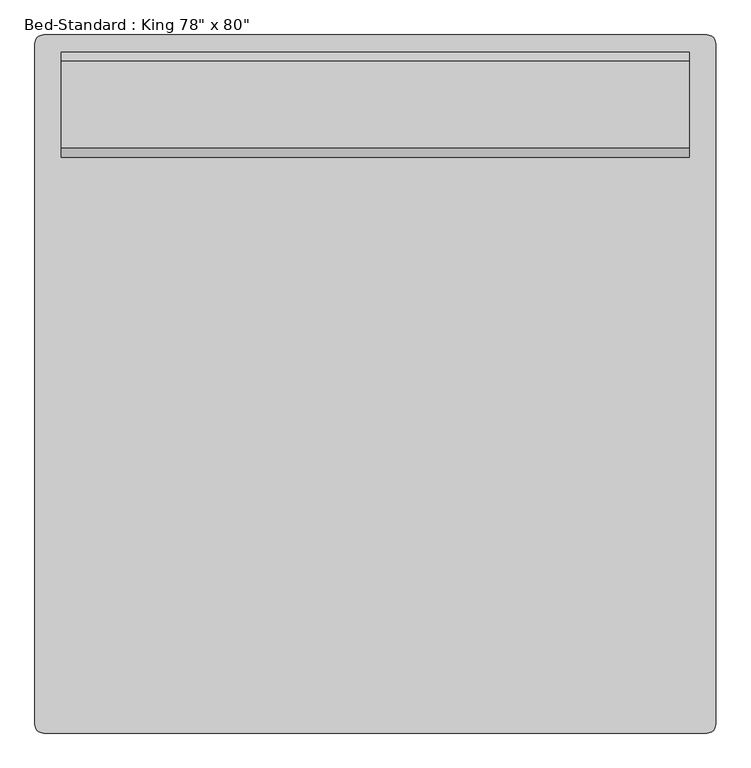
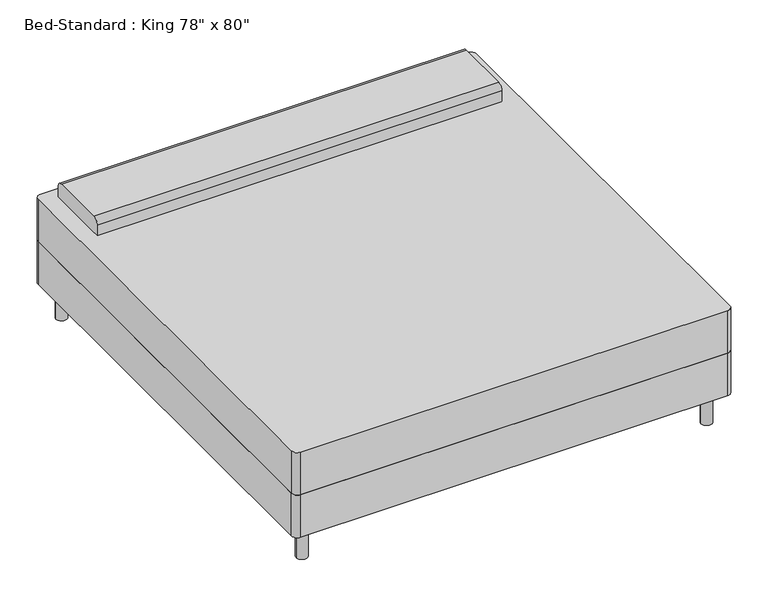
"""IFC4 building model written with IfcOpenShell, lengths in millimetres: furniture geometry."""

from ifc_helpers import new_model, si_unit, point, frame, frame_2d, origin, origin_with_axes, place, context, project, spatial, polyline, circle_curve, trimmed, segment, composite_curve, outline, extrude, source, transform, mapped, element, save


def furniture_1fc5af50(model_context):
    return source(origin(), model_context, "Body", "SweptSolid", [
        extrude(outline(composite_curve([segment(polyline([(-719.1114754, -1036.195082), (-719.1114754, 945.004918)]), True, "CONTINUOUS"), segment(trimmed(circle_curve(frame_2d((-693.7114754, 945.004918)), 25.4), [point((-719.1114754, 945.004918))], [point((-693.7114754, 970.404918))], False, "CARTESIAN"), True, "CONTINUOUS"), segment(polyline([(-693.7114754, 970.404918), (1236.6885246, 970.404918)]), True, "CONTINUOUS"), segment(trimmed(circle_curve(frame_2d((1236.6885246, 945.004918)), 25.4), [point((1236.6885246, 970.404918))], [point((1262.0885246, 945.004918))], False, "CARTESIAN"), True, "CONTINUOUS"), segment(polyline([(1262.0885246, 945.004918), (1262.0885246, -1036.195082)]), True, "CONTINUOUS"), segment(trimmed(circle_curve(frame_2d((1236.6885246, -1036.195082)), 25.4), [point((1262.0885246, -1036.195082))], [point((1236.6885246, -1061.595082))], False, "CARTESIAN"), True, "CONTINUOUS"), segment(polyline([(1236.6885246, -1061.595082), (-693.7114754, -1061.595082)]), True, "CONTINUOUS"), segment(trimmed(circle_curve(frame_2d((-693.7114754, -1036.195082)), 25.4), [point((-693.7114754, -1061.595082))], [point((-719.1114754, -1036.195082))], False, "CARTESIAN"), True, "CONTINUOUS")], self_intersect=False)), frame((0.0, 0.0, 152.4), z_axis=(0.0, 0.0, 1.0), x_axis=(1.0, 0.0, 0.0)), (0.0, 0.0, 1.0), 203.2),
        extrude(outline(composite_curve([segment(polyline([(614.804918, 558.8), (614.804918, 609.6)]), True, "CONTINUOUS"), segment(trimmed(circle_curve(frame_2d((640.204918, 609.6)), 25.4), [point((614.804918, 609.6))], [point((640.204918, 635.0))], False, "CARTESIAN"), True, "CONTINUOUS"), segment(polyline([(640.204918, 635.0), (894.204918, 635.0)]), True, "CONTINUOUS"), segment(trimmed(circle_curve(frame_2d((894.204918, 609.6)), 25.4), [point((894.204918, 635.0))], [point((919.604918, 609.6))], False, "CARTESIAN"), True, "CONTINUOUS"), segment(polyline([(919.604918, 609.6), (919.604918, 558.8), (614.804918, 558.8)]), True, "CONTINUOUS")], self_intersect=False)), frame((-642.9114754, 0.0, 0.0), z_axis=(1.0, 0.0, 0.0), x_axis=(0.0, 1.0, 0.0)), (0.0, 0.0, 1.0), 1828.8),
        extrude(outline(composite_curve([segment(trimmed(circle_curve(frame_2d((-642.9114754, 894.204918)), 25.4), [point((-668.3114754, 894.204918))], [point((-617.5114754, 894.204918))], False, "CARTESIAN"), True, "CONTINUOUS"), segment(trimmed(circle_curve(frame_2d((-642.9114754, 894.204918)), 25.4), [point((-617.5114754, 894.204918))], [point((-668.3114754, 894.204918))], False, "CARTESIAN"), True, "CONTINUOUS")], self_intersect=False)), origin_with_axes(), (0.0, 0.0, 1.0), 152.4),
        extrude(outline(composite_curve([segment(trimmed(circle_curve(frame_2d((1185.8885246, 894.204918)), 25.4), [point((1160.4885246, 894.204918))], [point((1211.2885246, 894.204918))], False, "CARTESIAN"), True, "CONTINUOUS"), segment(trimmed(circle_curve(frame_2d((1185.8885246, 894.204918)), 25.4), [point((1211.2885246, 894.204918))], [point((1160.4885246, 894.204918))], False, "CARTESIAN"), True, "CONTINUOUS")], self_intersect=False)), origin_with_axes(), (0.0, 0.0, 1.0), 152.4),
        extrude(outline(composite_curve([segment(trimmed(circle_curve(frame_2d((1185.8885246, -985.395082)), 25.4), [point((1160.4885246, -985.395082))], [point((1211.2885246, -985.395082))], False, "CARTESIAN"), True, "CONTINUOUS"), segment(trimmed(circle_curve(frame_2d((1185.8885246, -985.395082)), 25.4), [point((1211.2885246, -985.395082))], [point((1160.4885246, -985.395082))], False, "CARTESIAN"), True, "CONTINUOUS")], self_intersect=False)), origin_with_axes(), (0.0, 0.0, 1.0), 152.4),
        extrude(outline(composite_curve([segment(trimmed(circle_curve(frame_2d((-642.9114754, -985.395082)), 25.4), [point((-668.3114754, -985.395082))], [point((-617.5114754, -985.395082))], False, "CARTESIAN"), True, "CONTINUOUS"), segment(trimmed(circle_curve(frame_2d((-642.9114754, -985.395082)), 25.4), [point((-617.5114754, -985.395082))], [point((-668.3114754, -985.395082))], False, "CARTESIAN"), True, "CONTINUOUS")], self_intersect=False)), origin_with_axes(), (0.0, 0.0, 1.0), 152.4),
        extrude(outline(composite_curve([segment(polyline([(-693.7114754, 970.404918), (1236.6885246, 970.404918)]), True, "CONTINUOUS"), segment(trimmed(circle_curve(frame_2d((1236.6885246, 945.004918)), 25.4), [point((1236.6885246, 970.404918))], [point((1262.0885246, 945.004918))], False, "CARTESIAN"), True, "CONTINUOUS"), segment(polyline([(1262.0885246, 945.004918), (1262.0885246, -1036.195082)]), True, "CONTINUOUS"), segment(trimmed(circle_curve(frame_2d((1236.6885246, -1036.195082)), 25.4), [point((1262.0885246, -1036.195082))], [point((1236.6885246, -1061.595082))], False, "CARTESIAN"), True, "CONTINUOUS"), segment(polyline([(1236.6885246, -1061.595082), (-693.7114754, -1061.595082)]), True, "CONTINUOUS"), segment(trimmed(circle_curve(frame_2d((-693.7114754, -1036.195082)), 25.4), [point((-693.7114754, -1061.595082))], [point((-719.1114754, -1036.195082))], False, "CARTESIAN"), True, "CONTINUOUS"), segment(polyline([(-719.1114754, -1036.195082), (-719.1114754, 945.004918)]), True, "CONTINUOUS"), segment(trimmed(circle_curve(frame_2d((-693.7114754, 945.004918)), 25.4), [point((-719.1114754, 945.004918))], [point((-693.7114754, 970.404918))], False, "CARTESIAN"), True, "CONTINUOUS")], self_intersect=False)), frame((0.0, 0.0, 355.6), z_axis=(0.0, 0.0, 1.0), x_axis=(1.0, 0.0, 0.0)), (0.0, 0.0, 1.0), 203.2),
    ])


if __name__ == "__main__":
    model = new_model("IFC4")
    model_context = context("Model", 3, world=origin())
    ifc_project = project(units=[si_unit("LENGTHUNIT", "METRE", prefix="MILLI")], contexts=[model_context])
    site = spatial("IfcSite", under=ifc_project)
    building = spatial("IfcBuilding", under=site)
    placement = place(None, origin())
    furniture_shape = furniture_1fc5af50(model_context)
    element("IfcFurniture", 1, ObjectType="Bed-Standard : King 78\" x 80\"", at=placement, inside=building, context=model_context, shape_type="MappedRepresentation", body=[
        mapped(furniture_shape, transform((0.0, 0.0, 0.0), x_axis=(1.0, 0.0, 0.0), y_axis=(0.0, 1.0, 0.0), z_axis=(0.0, 0.0, 1.0))),
    ])
    save(model, "model.ifc")

# Revit data of these elements
# Type "Bed-Standard : King 78\" x 80\""
#   Assembly Code = "E2020200"
#   Length = 6' - 8"
#   Width = 6' - 6"
#   Leg Material = Steel, Chrome Plated
#   Mattress Material = Linen, White
#   Default Elevation = 0
# Element 1 (IfcFurniture, "Bed-Standard : King 78\" x 80\"")
#   Materials on its faces: "Linen, White", "Steel, Chrome Plated"
# Materials
#   "Steel, Chrome Plated": class "Metal", colour RGB 17 17 17, transparency 0, Description = "Chromiuim plated steel", Cost = 0
#   "Linen, White": class "Textile", colour RGB 247 247 239, transparency 0, Description = "Linen, white", Cost = 0
